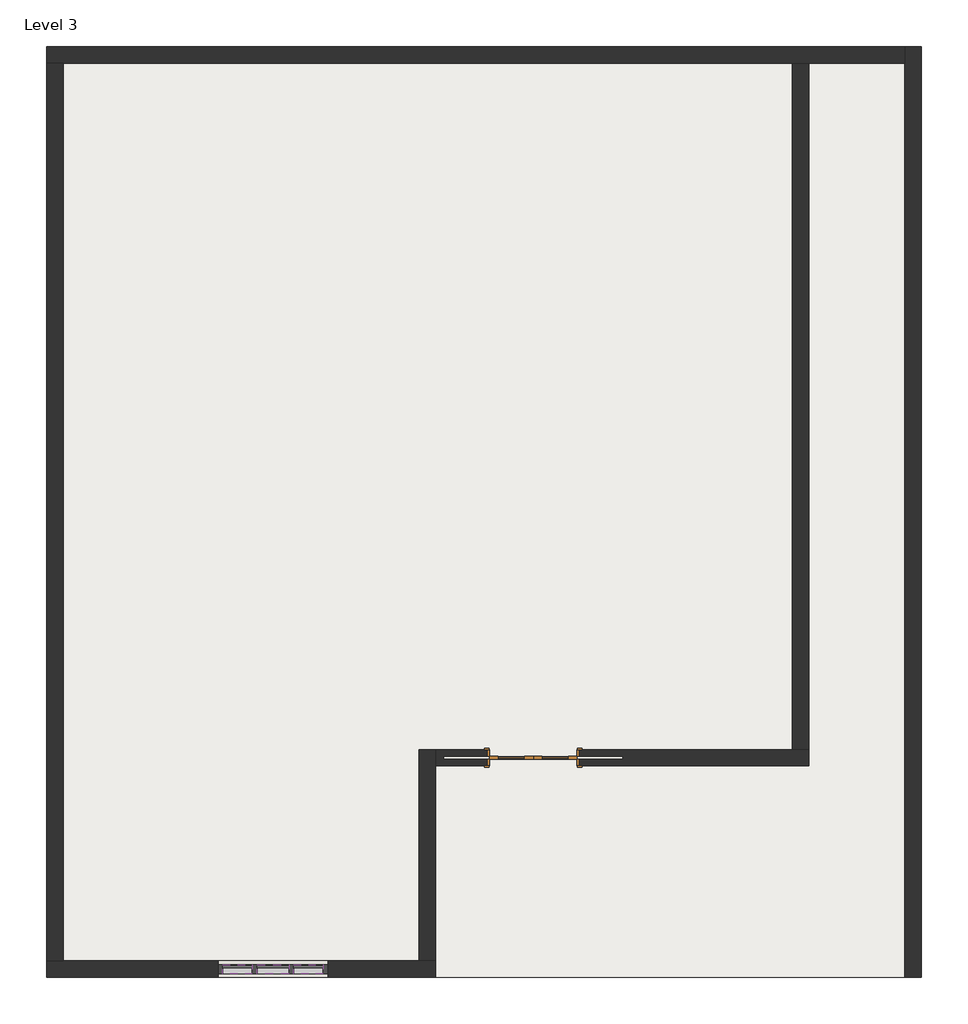
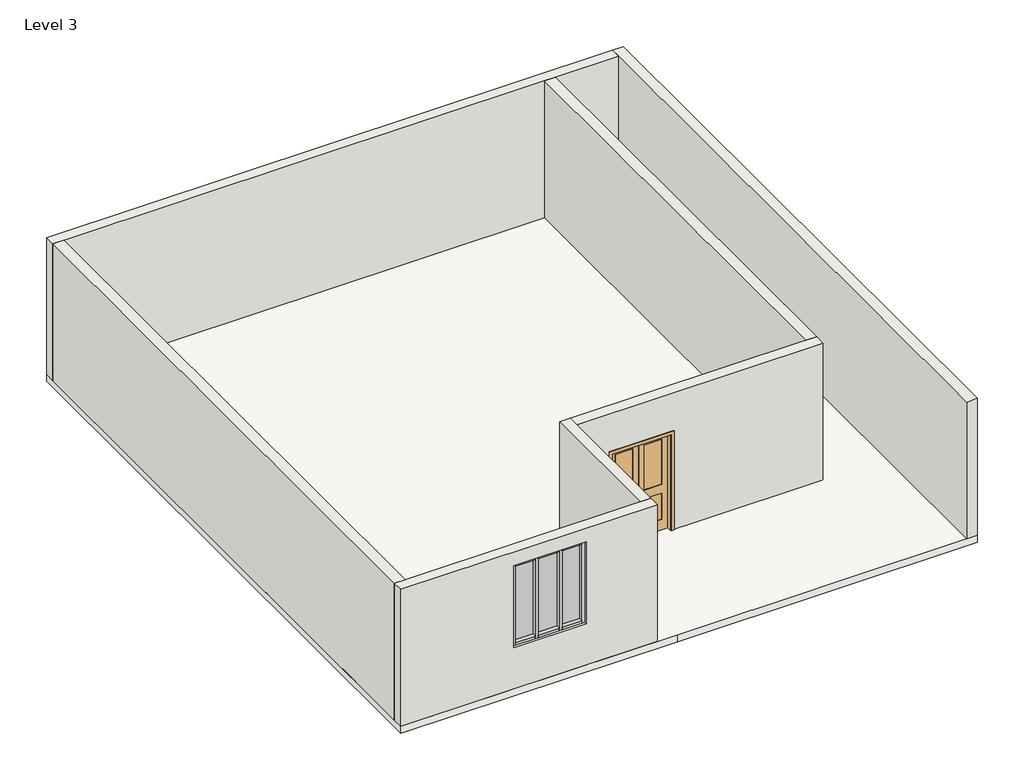
# One storey: 10 members, 7 walls, 3 plates, 1 door, 1 slab.
"""IFC4 building model written with IfcOpenShell, lengths in millimetres."""

from ifc_helpers import new_model, si_unit, frame, origin, place, context, project, spatial, polyline, outline, extrude, faceted_brep, transform, mapped, element, save
from components import door_interior_double_pocket_2_panel_wood_4_x7_3a565322, member_dc106669, member_d60e8053, member_bc7dbe04, member_2fae0574, system_panel_glazed_c73a426b, system_panel_glazed_693f0248

model = new_model("IFC4")

# Units and contexts
model_context = context("Model", 3, world=origin())
ifc_project = project(units=[si_unit("LENGTHUNIT", "METRE", prefix="MILLI")], contexts=[model_context])

# Site, building, storey
site = spatial("IfcSite", under=ifc_project)
building = spatial("IfcBuilding", under=site)
storey = spatial("IfcBuildingStorey", under=building, Name="Level 3", Elevation=3810.0)

# Door
placement = place(None, origin())
door_interior_double_pocket_2_panel_wood_4_x7_shape = door_interior_double_pocket_2_panel_wood_4_x7_3a565322(model_context)
element("IfcDoor", 1, ObjectType="Door-Interior-Double-Pocket-2_Panel-Wood : 4'x7'", at=placement, inside=storey, context=model_context, shape_type="MappedRepresentation", body=[
    mapped(door_interior_double_pocket_2_panel_wood_4_x7_shape, transform((-3028.8540309, 3243.2033856, 3810.0), x_axis=(-1.0, 0.0, 0.0), y_axis=(0.0, -1.0, 0.0), z_axis=(0.0, 0.0, 1.0))),
])

# Members
member_shape = member_dc106669(model_context)
element("IfcMember", 2, ObjectType="Rectangular Mullion : 2.5\" x 5\" rectangular", at=placement, inside=storey, context=model_context, shape_type="MappedRepresentation", body=[
    mapped(member_shape, transform((-5943.5040309, 309.5033856, 6553.2), x_axis=(0.0, 0.0, 1.0), y_axis=(0.0, -1.0, 0.0), z_axis=(1.0, 0.0, 0.0))),
])
element("IfcMember", 3, ObjectType="Rectangular Mullion : 2.5\" x 5\" rectangular", at=placement, inside=storey, context=model_context, shape_type="MappedRepresentation", body=[
    mapped(member_shape, transform((-6927.7540309, 309.5033856, 6553.2), x_axis=(0.0, 0.0, 1.0), y_axis=(0.0, -1.0, 0.0), z_axis=(1.0, 0.0, 0.0))),
])
element("IfcMember", 4, ObjectType="Rectangular Mullion : 2.5\" x 5\" rectangular", at=placement, inside=storey, context=model_context, shape_type="MappedRepresentation", body=[
    mapped(member_shape, transform((-7340.5040309, 309.5033856, 4724.4), x_axis=(0.0, 0.0, -1.0), y_axis=(0.0, -1.0, 0.0), z_axis=(-1.0, 0.0, 0.0))),
])
element("IfcMember", 5, ObjectType="Rectangular Mullion : 2.5\" x 5\" rectangular", at=placement, inside=storey, context=model_context, shape_type="MappedRepresentation", body=[
    mapped(member_shape, transform((-6356.2540309, 309.5033856, 4724.4), x_axis=(0.0, 0.0, -1.0), y_axis=(0.0, -1.0, 0.0), z_axis=(-1.0, 0.0, 0.0))),
])
member_2_shape = member_d60e8053(model_context)
element("IfcMember", 6, ObjectType="Rectangular Mullion : 2.5\" x 5\" rectangular", at=placement, inside=storey, context=model_context, shape_type="MappedRepresentation", body=[
    mapped(member_2_shape, transform((-6896.0040309, 309.5033856, 4724.4), x_axis=(1.0, 0.0, 0.0), y_axis=(0.0, -1.0, 0.0), z_axis=(0.0, 0.0, -1.0))),
])
element("IfcMember", 7, ObjectType="Rectangular Mullion : 2.5\" x 5\" rectangular", at=placement, inside=storey, context=model_context, shape_type="MappedRepresentation", body=[
    mapped(member_2_shape, transform((-6388.0040309, 309.5033856, 4724.4), x_axis=(1.0, 0.0, 0.0), y_axis=(0.0, -1.0, 0.0), z_axis=(0.0, 0.0, -1.0))),
])
member_3_shape = member_bc7dbe04(model_context)
element("IfcMember", 8, ObjectType="Rectangular Mullion : 2.5\" x 5\" rectangular", at=placement, inside=storey, context=model_context, shape_type="MappedRepresentation", body=[
    mapped(member_3_shape, transform((-6864.2540309, 309.5033856, 4724.4), x_axis=(0.0, 0.0, -1.0), y_axis=(0.0, -1.0, 0.0), z_axis=(-1.0, 0.0, 0.0))),
])
element("IfcMember", 9, ObjectType="Rectangular Mullion : 2.5\" x 5\" rectangular", at=placement, inside=storey, context=model_context, shape_type="MappedRepresentation", body=[
    mapped(member_3_shape, transform((-6419.7540309, 309.5033856, 6553.2), x_axis=(0.0, 0.0, 1.0), y_axis=(0.0, -1.0, 0.0), z_axis=(1.0, 0.0, 0.0))),
])
member_4_shape = member_2fae0574(model_context)
element("IfcMember", 10, ObjectType="Rectangular Mullion : 2.5\" x 5\" rectangular", at=placement, inside=storey, context=model_context, shape_type="MappedRepresentation", body=[
    mapped(member_4_shape, transform((-7404.0040309, 309.5033856, 6553.2), x_axis=(-1.0, 0.0, 0.0), y_axis=(0.0, -1.0, 0.0), z_axis=(0.0, 0.0, 1.0))),
])
element("IfcMember", 11, ObjectType="Rectangular Mullion : 2.5\" x 5\" rectangular", at=placement, inside=storey, context=model_context, shape_type="MappedRepresentation", body=[
    mapped(member_4_shape, transform((-5880.0040309, 309.5033856, 4724.4), x_axis=(1.0, 0.0, 0.0), y_axis=(0.0, -1.0, 0.0), z_axis=(0.0, 0.0, -1.0))),
])

# Plates
system_panel_glazed_shape = system_panel_glazed_c73a426b(model_context)
element("IfcPlate", 12, ObjectType="System Panel : Glazed", at=placement, inside=storey, context=model_context, shape_type="MappedRepresentation", body=[
    mapped(system_panel_glazed_shape, transform((-7134.1290309, 309.5033856, 4787.9), x_axis=(1.0, 0.0, 0.0), y_axis=(0.0, 1.0, 0.0), z_axis=(0.0, 0.0, 1.0))),
])
element("IfcPlate", 13, ObjectType="System Panel : Glazed", at=placement, inside=storey, context=model_context, shape_type="MappedRepresentation", body=[
    mapped(system_panel_glazed_shape, transform((-6149.8790309, 309.5033856, 4787.9), x_axis=(1.0, 0.0, 0.0), y_axis=(0.0, 1.0, 0.0), z_axis=(0.0, 0.0, 1.0))),
])
system_panel_glazed_2_shape = system_panel_glazed_693f0248(model_context)
element("IfcPlate", 14, ObjectType="System Panel : Glazed", at=placement, inside=storey, context=model_context, shape_type="MappedRepresentation", body=[
    mapped(system_panel_glazed_2_shape, transform((-6642.0040309, 309.5033856, 4787.9), x_axis=(1.0, 0.0, 0.0), y_axis=(0.0, 1.0, 0.0), z_axis=(0.0, 0.0, 1.0))),
])

# Slab
element("IfcSlab", 15, ObjectType="6\"", at=placement, inside=storey, context=model_context, shape_type="SweptSolid", body=[
    extrude(outline(polyline([(-9785.2540309, 13111.1033856), (2355.9459691, 13111.1033856), (2355.9459691, 195.2033856), (-3955.9540309, 195.2033856), (-9785.2540309, 195.2033856), (-9785.2540309, 13111.1033856)])), frame((0.0, 0.0, 3657.6), z_axis=(0.0, 0.0, 1.0), x_axis=(1.0, 0.0, 0.0)), (0.0, 0.0, 1.0), 152.4),
])

# Walls
element("IfcWall", 16, ObjectType="9\" wall", at=placement, inside=storey, context=model_context, shape_type="Brep", body=[
    faceted_brep([(-9785.2540309, 12882.5033856, 3810.0), (-9556.6540309, 12882.5033856, 3810.0), (565.2459691, 12882.5033856, 3810.0), (793.8459691, 12882.5033856, 3810.0), (2127.3459691, 12882.5033856, 3810.0), (2127.3459691, 12882.5033856, 6858.0), (793.8459691, 12882.5033856, 6858.0), (565.2459691, 12882.5033856, 6858.0), (-9556.6540309, 12882.5033856, 6858.0), (-9785.2540309, 12882.5033856, 6858.0), (-9785.2540309, 13111.1033856, 3810.0), (-9785.2540309, 13111.1033856, 6858.0), (2127.3459691, 13111.1033856, 6858.0), (2127.3459691, 13111.1033856, 3810.0)], [[[0, 1, 2, 3, 4, 5, 6, 7, 8, 9]], [[10, 11, 12, 13]], [[4, 3, 2, 1, 0, 10, 13]], [[9, 8, 7, 6, 5, 12, 11]], [[0, 9, 11, 10]], [[5, 4, 13, 12]]]),
])
element("IfcWall", 17, ObjectType="9\" wall", at=placement, inside=storey, context=model_context, shape_type="Brep", body=[
    faceted_brep([(2127.3459691, 13111.1033856, 3810.0), (2127.3459691, 12882.5033856, 3810.0), (2127.3459691, 195.2033856, 3810.0), (2127.3459691, 195.2033856, 6858.0), (2127.3459691, 12882.5033856, 6858.0), (2127.3459691, 13111.1033856, 6858.0), (2355.9459691, 13111.1033856, 3810.0), (2355.9459691, 13111.1033856, 6858.0), (2355.9459691, 195.2033856, 6858.0), (2355.9459691, 195.2033856, 3810.0)], [[[0, 1, 2, 3, 4, 5]], [[6, 7, 8, 9]], [[2, 1, 0, 6, 9]], [[3, 2, 9, 8]], [[5, 4, 3, 8, 7]], [[0, 5, 7, 6]]]),
])
element("IfcWall", 18, ObjectType="9\" wall", at=placement, inside=storey, context=model_context, shape_type="Brep", body=[
    faceted_brep([(793.8459691, 3128.9033856, 6858.0), (-4387.7540309, 3128.9033856, 6858.0), (-4387.7540309, 3128.9033856, 3810.0), (-3663.8540309, 3128.9033856, 3810.0), (-3663.8540309, 3128.9033856, 5969.0), (-2393.8540309, 3128.9033856, 5969.0), (-2393.8540309, 3128.9033856, 3810.0), (793.8459691, 3128.9033856, 3810.0), (-4387.7540309, 3357.5033856, 6858.0), (565.2459691, 3357.5033856, 6858.0), (793.8459691, 3357.5033856, 6858.0), (793.8459691, 3357.5033856, 3810.0), (565.2459691, 3357.5033856, 3810.0), (-2393.8540309, 3357.5033856, 3810.0), (-2393.8540309, 3357.5033856, 5969.0), (-3663.8540309, 3357.5033856, 5969.0), (-3663.8540309, 3357.5033856, 3810.0), (-4387.7540309, 3357.5033856, 3810.0), (-3663.8540309, 3263.8408856, 3810.0), (-4273.4540309, 3263.8408856, 3810.0), (-4273.4540309, 3222.5658856, 3810.0), (-3663.8540309, 3222.5658856, 3810.0), (-2393.8540309, 3222.5658856, 3810.0), (-1784.2540309, 3222.5658856, 3810.0), (-1784.2540309, 3263.8408856, 3810.0), (-2393.8540309, 3263.8408856, 3810.0), (-4273.4540309, 3222.5658856, 5969.0), (-4273.4540309, 3263.8408856, 5969.0), (-3663.8540309, 3263.8408856, 5969.0), (-2393.8540309, 3263.8408856, 5969.0), (-1784.2540309, 3263.8408856, 5969.0), (-1784.2540309, 3222.5658856, 5969.0), (-2393.8540309, 3222.5658856, 5969.0), (-3663.8540309, 3222.5658856, 5969.0)], [[[0, 1, 2, 3, 4, 5, 6, 7]], [[8, 9, 10, 11, 12, 13, 14, 15, 16, 17]], [[2, 17, 16, 18, 19, 20, 21, 3]], [[11, 7, 6, 22, 23, 24, 25, 13, 12]], [[1, 0, 10, 9, 8]], [[2, 1, 8, 17]], [[26, 27, 28, 15, 14, 29, 30, 31, 32, 5, 4, 33]], [[26, 33, 21, 20]], [[33, 4, 3, 21]], [[5, 32, 22, 6]], [[32, 31, 23, 22]], [[31, 30, 24, 23]], [[30, 29, 25, 24]], [[29, 14, 13, 25]], [[15, 28, 18, 16]], [[28, 27, 19, 18]], [[27, 26, 20, 19]], [[0, 7, 11, 10]]]),
])
element("IfcWall", 19, ObjectType="9\" wall", at=placement, inside=storey, context=model_context, shape_type="Brep", body=[
    faceted_brep([(-4387.7540309, 423.8033856, 3810.0), (-4616.3540309, 423.8033856, 3810.0), (-9556.6540309, 423.8033856, 3810.0), (-9785.2540309, 423.8033856, 3810.0), (-9785.2540309, 423.8033856, 6858.0), (-9556.6540309, 423.8033856, 6858.0), (-4616.3540309, 423.8033856, 6858.0), (-4387.7540309, 423.8033856, 6858.0), (-7404.0040309, 423.8033856, 6553.2), (-7404.0040309, 423.8033856, 4724.4), (-5880.0040309, 423.8033856, 4724.4), (-5880.0040309, 423.8033856, 6553.2), (-9785.2540309, 195.2033856, 3810.0), (-4387.7540309, 195.2033856, 3810.0), (-4387.7540309, 195.2033856, 6858.0), (-9785.2540309, 195.2033856, 6858.0), (-7404.0040309, 195.2033856, 4724.4), (-7404.0040309, 195.2033856, 6553.2), (-5880.0040309, 195.2033856, 6553.2), (-5880.0040309, 195.2033856, 4724.4)], [[[0, 1, 2, 3, 4, 5, 6, 7], [8, 9, 10, 11]], [[12, 13, 14, 15], [16, 17, 18, 19]], [[3, 2, 1, 0, 13, 12]], [[7, 6, 5, 4, 15, 14]], [[4, 3, 12, 15]], [[0, 7, 14, 13]], [[16, 9, 8, 17]], [[17, 8, 11, 18]], [[18, 11, 10, 19]], [[9, 16, 19, 10]]]),
])
element("IfcWall", 20, ObjectType="9\" wall", at=placement, inside=storey, context=model_context, shape_type="SweptSolid", body=[
    extrude(outline(polyline([(-9556.6540309, 12882.5033856), (-9556.6540309, 423.8033856), (-9785.2540309, 423.8033856), (-9785.2540309, 12882.5033856), (-9556.6540309, 12882.5033856)])), frame((0.0, 0.0, 3810.0), z_axis=(0.0, 0.0, 1.0), x_axis=(1.0, 0.0, 0.0)), (0.0, 0.0, 1.0), 3048.0),
])
element("IfcWall", 21, ObjectType="9\" wall", at=placement, inside=storey, context=model_context, shape_type="Brep", body=[
    faceted_brep([(-4387.7540309, 423.8033856, 3810.0), (-4387.7540309, 3128.9033856, 3810.0), (-4387.7540309, 3357.5033856, 3810.0), (-4387.7540309, 3357.5033856, 6858.0), (-4387.7540309, 3128.9033856, 6858.0), (-4387.7540309, 423.8033856, 6858.0), (-4616.3540309, 423.8033856, 3810.0), (-4616.3540309, 423.8033856, 6858.0), (-4616.3540309, 3357.5033856, 6858.0), (-4616.3540309, 3357.5033856, 3810.0)], [[[0, 1, 2, 3, 4, 5]], [[6, 7, 8, 9]], [[2, 1, 0, 6, 9]], [[5, 4, 3, 8, 7]], [[3, 2, 9, 8]], [[0, 5, 7, 6]]]),
])
element("IfcWall", 22, ObjectType="9\" wall", at=placement, inside=storey, context=model_context, shape_type="SweptSolid", body=[
    extrude(outline(polyline([(793.8459691, 12882.5033856), (793.8459691, 3357.5033856), (565.2459691, 3357.5033856), (565.2459691, 12882.5033856), (793.8459691, 12882.5033856)])), frame((0.0, 0.0, 3810.0), z_axis=(0.0, 0.0, 1.0), x_axis=(1.0, 0.0, 0.0)), (0.0, 0.0, 1.0), 3048.0),
])

save(model, "model.ifc")

# Revit data of these elements
# Type "Door-Interior-Double-Pocket-2_Panel-Wood : 4'x7'"
#   Type Mark = "9"
#   Assembly Code = "C1020300"
#   Analytic Construction = "Wooden"
#   Top Rail = 0' - 4 11/16"
#   Thickness = 0' - 1 3/8"
#   Thermal Resistance (R) = 2.5876 (h·ft²·°F)/BTU
#   Stiles = 0' - 4 3/4"
#   Rough Width = 8' - 2"
#   Rough Height = 7' - 4 1/2"
#   Panel Width = 2' - 0"
#   Lock Rail = 0' - 7 1/2"
#   Location [instance default] = 2' - 1"
#   Height = 7' - 0"
#   Width = 4' - 0"
#   Heat Transfer Coefficient (U) = 0.3865 BTU/(h·ft²·°F)
#   Bottom Rail = 0' - 9 1/8"
#   Panel Open [instance default] = no
#   Trim Material = Cherry
#   Panel Material = Cherry
#   Frame Material = Cherry
#   Visual Light Transmittance = 0
#   Solar Heat Gain Coefficient = 0
#   Wall Closure = (empty or 0)
#   Function = (empty or 0)
# Type "Rectangular Mullion : 2.5\" x 5\" rectangular"
#   built-in parameter 1007304 = 0.416667 (stored number, unit not read)
#   built-in parameter 1007301 = 0.104167 (stored number, unit not read)
#   built-in parameter 1007300 = 0.104167 (stored number, unit not read)
# Type "System Panel : Glazed"
#   Construction Type Id = "GSP4R"
#   Analytic Construction = "1/8 in Pilkington single glazing"
#   Visual Light Transmittance = 0.9
#   Solar Heat Gain Coefficient = 0.86
#   Heat Transfer Coefficient (U) = 1.18115 BTU/(h·ft²·°F)
#   Define Thermal Properties by = 1
# Type "6\""
#   Assembly Code = "B1010"
#   Function = 0
#   Layers, outside or top first: 0' - 6" "Gypsum Wall Board" (function 1)
# Type "9\" wall"
#   Assembly Code = "B2010"
#   Layers, outside or top first: 0' - 9" "Gypsum Wall Board" (function 1)
# Element 1 (IfcDoor, "Door-Interior-Double-Pocket-2_Panel-Wood : 4'x7'")
#   Location = 2' - 1"
#   Panel Open = no
#   Phase Created = New Construction
#   Materials on its faces: "Cherry"
# Elements 2, 3, 4, 5, 6, 7, 8, 9, 10, 11 (IfcMember, "Rectangular Mullion : 2.5\" x 5\" rectangular")
#   Phase Created = New Construction
# Elements 12, 13, 14 (IfcPlate, "System Panel : Glazed")
#   Phase Created = New Construction
#   Materials on its faces: "Glass"
# Element 15 (IfcSlab, "6\"")
#   built-in parameter 1001955 = 3.14159 (stored number, unit not read)
#   Height Offset From Level = 0' - 0"
#   Phase Created = New Construction
#   Materials on its faces: "Gypsum Wall Board"
# Elements 16, 17, 18, 19, 20, 21, 22 (IfcWall, "9\" wall")
#   Top Offset = 0' - 0"
#   Base Offset = 0' - 0"
#   wall height = 10' - 0"
#   Phase Created = New Construction
#   Base Constraint = Level 3
#   Top Constraint = Level 4
#   Materials on its faces: "Gypsum Wall Board"
# Materials
#   "Cherry": class "Wood", colour RGB 226 177 128, transparency 0, Description = "Prunus Serotina", Cost = 0
#   "Gypsum Wall Board": class "Generic", colour RGB 127 127 127, transparency 0, Description = "Gypsum Wall Board", Cost = 0
#   "Glass": class "Glass", colour RGB 0 128 192, transparency 0.75, Description = "Soda Lime Glass", Cost = 0
